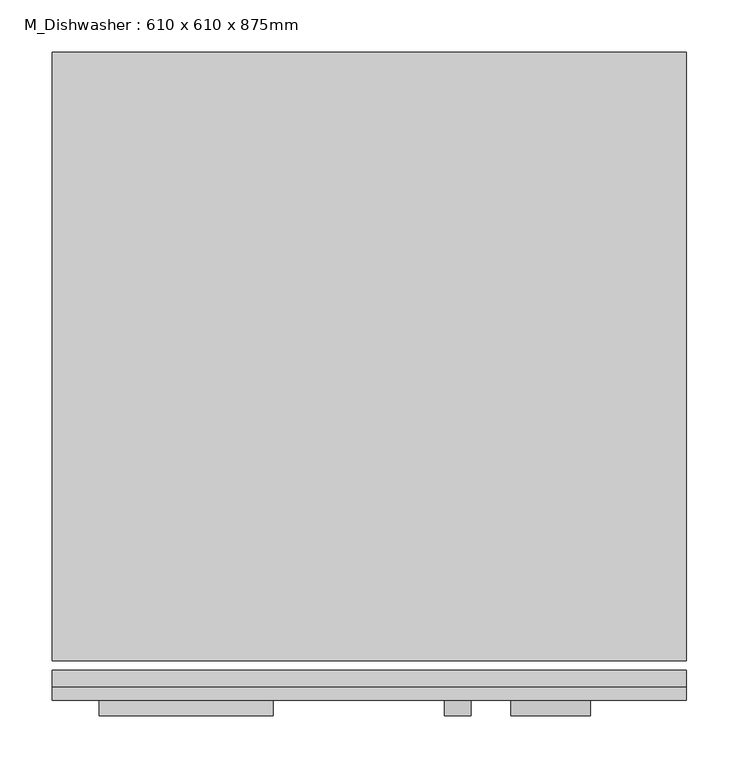
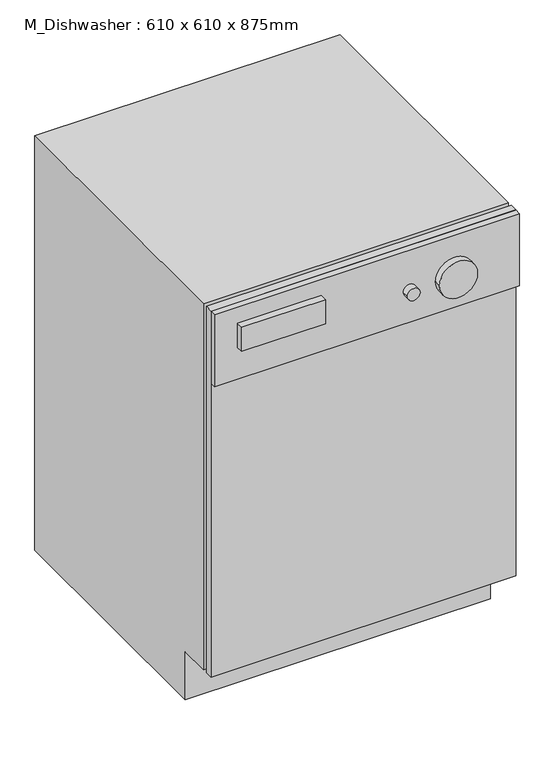
"""IFC4 building model written with IfcOpenShell, lengths in millimetres: proxy geometry, M_Dishwasher : 610 x 610 x 875mm."""

from ifc_helpers import new_model, si_unit, point, frame, frame_2d, origin, place, context, project, spatial, polyline, circle_curve, trimmed, segment, composite_curve, outline, extrude, source, transform, mapped, element, save


def m_dishwasher_610_x_610_x_875mm_54ecfc4c(model_context):
    return source(origin(), model_context, "Body", "SweptSolid", [
        extrude(outline(polyline([(687.5174685, -38.3504352), (77.5174685, -38.3504352), (77.5174685, -22.4754352), (687.5174685, -22.4754352), (687.5174685, -38.3504352)])), frame((0.0, 0.0, 101.6), z_axis=(0.0, 0.0, 1.0), x_axis=(1.0, 0.0, 0.0)), (0.0, 0.0, 1.0), 773.4),
        extrude(outline(polyline([(687.5174685, -38.3504352), (687.5174685, -51.0504352), (77.5174685, -51.0504352), (77.5174685, -38.3504352), (687.5174685, -38.3504352)])), frame((0.0, 0.0, 722.6), z_axis=(0.0, 0.0, 1.0), x_axis=(1.0, 0.0, 0.0)), (0.0, 0.0, 1.0), 152.4),
        extrude(outline(polyline([(571.6495648, 0.0), (50.5495648, 0.0), (50.5495648, 101.6), (-12.9504352, 101.6), (-12.9504352, 875.0), (571.6495648, 875.0), (571.6495648, 0.0)])), frame((77.5174685, 0.0, 0.0), z_axis=(1.0, 0.0, 0.0), x_axis=(0.0, 1.0, 0.0)), (0.0, 0.0, 1.0), 610.0),
        extrude(outline(polyline([(290.2347603, -66.0504352), (122.8347603, -66.0504352), (122.8347603, -51.0504352), (290.2347603, -51.0504352), (290.2347603, -66.0504352)])), frame((0.0, 0.0, 790.6663551), z_axis=(0.0, 0.0, 1.0), x_axis=(1.0, 0.0, 0.0)), (0.0, 0.0, 1.0), 50.8),
        extrude(outline(composite_curve([segment(trimmed(circle_curve(frame_2d((790.6663551, 467.3393328)), 12.7), [point((790.6663551, 480.0393328))], [point((790.6663551, 454.6393328))], False, "CARTESIAN"), True, "CONTINUOUS"), segment(trimmed(circle_curve(frame_2d((790.6663551, 467.3393328)), 12.7), [point((790.6663551, 454.6393328))], [point((790.6663551, 480.0393328))], False, "CARTESIAN"), True, "CONTINUOUS")], self_intersect=False)), frame((0.0, -66.0504352, 0.0), z_axis=(0.0, 1.0, 0.0), x_axis=(0.0, 0.0, 1.0)), (0.0, 0.0, 1.0), 15.0),
        extrude(outline(composite_curve([segment(trimmed(circle_curve(frame_2d((790.6663551, 556.7855874)), 38.1), [point((790.6663551, 594.8855874))], [point((790.6663551, 518.6855874))], False, "CARTESIAN"), True, "CONTINUOUS"), segment(trimmed(circle_curve(frame_2d((790.6663551, 556.7855874)), 38.1), [point((790.6663551, 518.6855874))], [point((790.6663551, 594.8855874))], False, "CARTESIAN"), True, "CONTINUOUS")], self_intersect=False)), frame((0.0, -66.0504352, 0.0), z_axis=(0.0, 1.0, 0.0), x_axis=(0.0, 0.0, 1.0)), (0.0, 0.0, 1.0), 15.0),
    ])


if __name__ == "__main__":
    model = new_model("IFC4")
    model_context = context("Model", 3, world=origin())
    ifc_project = project(units=[si_unit("LENGTHUNIT", "METRE", prefix="MILLI")], contexts=[model_context])
    site = spatial("IfcSite", under=ifc_project)
    building = spatial("IfcBuilding", under=site)
    placement = place(None, origin())
    m_dishwasher_610_x_610_x_875mm_shape = m_dishwasher_610_x_610_x_875mm_54ecfc4c(model_context)
    element("IfcBuildingElementProxy", 1, Name="M_Dishwasher : 610 x 610 x 875mm", ObjectType="M_Dishwasher : 610 x 610 x 875mm", at=placement, inside=building, context=model_context, shape_type="MappedRepresentation", body=[
        mapped(m_dishwasher_610_x_610_x_875mm_shape, transform((0.0, 0.0, 0.0), x_axis=(1.0, 0.0, 0.0), y_axis=(0.0, 1.0, 0.0), z_axis=(0.0, 0.0, 1.0))),
    ])
    save(model, "model.ifc")

# Revit data of these elements
# Type "M_Dishwasher : 610 x 610 x 875mm"
#   Label = "DW"
#   Depth = 610 mm
#   Height = 875 mm
#   Width = 610 mm
#   Dishwasher Material = Steel, Paint Finish, Ivory, Glossy
#   Panel Face Material = Plastic, Opaque Black
#   Default Elevation = 0
# Element 1 (IfcBuildingElementProxy, "M_Dishwasher : 610 x 610 x 875mm")
#   Materials on its faces: "Steel, Paint Finish, Ivory, Glossy", "Plastic, Opaque Black"
# Materials
#   "Steel, Paint Finish, Ivory, Glossy": class "Metal", colour RGB 247 247 239, transparency 0, Description = "Steel, paint finish, ivory, glossy", Cost = 0
#   "Plastic, Opaque Black": class "Plastic", colour RGB 0 0 0, transparency 0.7, Description = "Plastic, generic, opaque black", Cost = 0
